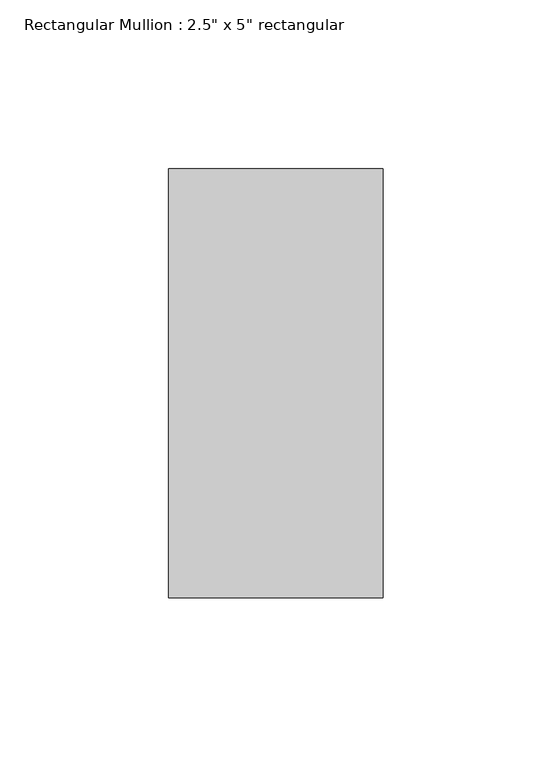
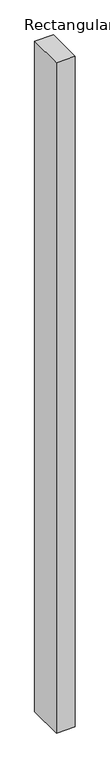
"""IFC4 building model written with IfcOpenShell, lengths in millimetres: member geometry."""

from ifc_helpers import new_model, si_unit, frame, origin, place, context, project, spatial, polyline, outline, extrude, source, transform, mapped, element, save


def member_c92b576d(model_context):
    return source(origin(), model_context, "Body", "SweptSolid", [
        extrude(outline(polyline([(0.0, 63.5), (0.0, -63.5), (-63.5, -63.5), (-63.5, 63.5), (0.0, 63.5)])), frame((0.0, 0.0, -2398.3558723), z_axis=(0.0, 0.0, 1.0), x_axis=(1.0, 0.0, 0.0)), (0.0, 0.0, 1.0), 2398.3558723),
    ])


if __name__ == "__main__":
    model = new_model("IFC4")
    model_context = context("Model", 3, world=origin())
    ifc_project = project(units=[si_unit("LENGTHUNIT", "METRE", prefix="MILLI")], contexts=[model_context])
    site = spatial("IfcSite", under=ifc_project)
    building = spatial("IfcBuilding", under=site)
    placement = place(None, origin())
    member_shape = member_c92b576d(model_context)
    element("IfcMember", 1, ObjectType="Rectangular Mullion : 2.5\" x 5\" rectangular", at=placement, inside=building, context=model_context, shape_type="MappedRepresentation", body=[
        mapped(member_shape, transform((0.0, 0.0, 0.0), x_axis=(1.0, 0.0, 0.0), y_axis=(0.0, 1.0, 0.0), z_axis=(0.0, 0.0, 1.0))),
    ])
    save(model, "model.ifc")

# Revit data of these elements
# Type "Rectangular Mullion : 2.5\" x 5\" rectangular"
#   built-in parameter 1007304 = 0.416667 (stored number, unit not read)
#   built-in parameter 1007301 = 0.104167 (stored number, unit not read)
#   built-in parameter 1007300 = 0.104167 (stored number, unit not read)
# Element 1 (IfcMember, "Rectangular Mullion : 2.5\" x 5\" rectangular")
#   Materials on its faces: "Aluminum"
# Materials
#   "Aluminum": class "Metal", colour RGB 247 247 247, transparency 0, Description = "Aluminum 6061", Cost = 0
